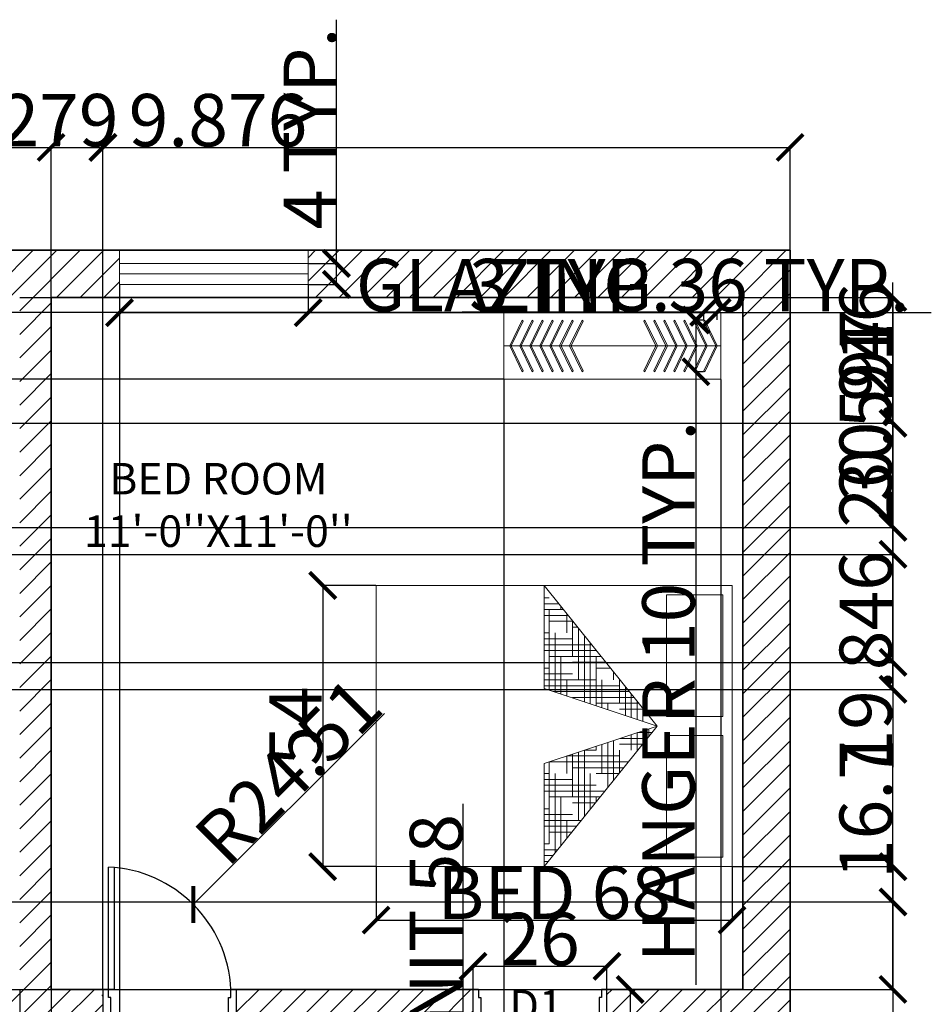
# Model space of a CAD drawing. Units: inches. Extents: x 90933 to 91345, y 21207 to 21646.
# Tile 4 of 4: x 91160 to 91334, y 21458 to 21646. Entities that reach past the tile are written whole.
import ezdxf

# ---------------------------------------------------------------- set-up
doc = ezdxf.new("R2010")
doc.units = ezdxf.units.IN
for name, color, linetype, lineweight in [('A-ANNO-DIMS', 2, 'Continuous', 18), ('A-ANNO-TEXT', 7, 'Continuous', 18), ('A-AREA-IDEN', 7, 'Continuous', 25), ('A-WALL-PATT', 8, 'Continuous', 13), ('B-FURNITURE', 9, 'Continuous', 18), ('Doors', 34, 'Continuous', 25), ('shelves', 42, 'Continuous', 18), ('Walls', 7, 'Continuous', 35), ('Windows', 140, 'Continuous', 18)]:
    doc.layers.add(name, color=color, linetype=linetype, lineweight=lineweight)
doc.styles.get("Standard").update_dxf_attribs({"font": 'arial.ttf'})
doc.dimstyles.get("Standard").update_dxf_attribs({"dimtxt": 10, "dimasz": 5, "dimexe": 0.18, "dimexo": 0.0625, "dimgap": 0.09, "dimtad": 1, "dimdec": 1, "dimzin": 0, "dimdsep": 46, "dimlunit": 4, "dimtxsty": 'Standard', "dimblk": 'ARCHTICK', "dimcen": 0.09, "dimadec": 0, "dimazin": 0, "dimtfac": 1, "dimtdec": 1, "dimtofl": 0, "dimtmove": 0, "dimatfit": 3, "dimldrblk": 'NONE', "dimfxl": 1, "dimtolj": 1, "dimtzin": 0, "dimarcsym": 0})

# ---------------------------------------------------------------- blocks, each defined once
blk = doc.blocks.new('*X5')
at = {"color": 0}
for p, q in [((20.1875, 14.75), (20.1875, 14.7669)), ((20.199, 14.7812), (20.2772, 14.7812)), ((20.25, 14.8125), (20.2772, 14.8125)), ((20.1487, 14.7188), (20.2772, 14.7188)), ((20.1562, 14.625), (20.1562, 14.7281)), ((20.1739, 14.75), (20.2772, 14.75)), ((20.25, 14.3194), (20.25, 14.75)), ((20.0984, 14.6562), (20.125, 14.6562)), ((20.1236, 14.6875), (20.25, 14.6875)), ((20.125, 14.5), (20.125, 14.6893)), ((20.0625, 14.2573), (20.0625, 14.6116)), ((20.0938, 14.375), (20.0938, 14.6504)), ((20.2188, 14.3091), (20.2188, 14.625)), ((20.25, 14.625), (20.2772, 14.625)), ((20.023, 14.5625), (20.2772, 14.5625)), ((20.0312, 14.2469), (20.0312, 14.5727)), ((20.125, 14.5938), (20.2772, 14.5938)), ((19.9727, 14.5), (20.25, 14.5)), ((19.9979, 14.5312), (20.2772, 14.5312)), ((20, 14.2366), (20, 14.5)), ((20.1875, 14.2987), (20.1875, 14.5)), ((19.9476, 14.4688), (20.125, 14.4688)), ((19.9062, 14.375), (19.9062, 14.4174)), ((19.9225, 14.4375), (20, 14.4375)), ((20.125, 14.4062), (20.2772, 14.4062)), ((20.25, 14.4375), (20.2772, 14.4375)), ((19.875, 14.25), (19.875, 14.3785)), ((19.875, 14.3438), (20.2772, 14.3438)), ((19.9688, 14.2262), (19.9688, 14.375)), ((20, 14.375), (20.2772, 14.375)), ((20.1562, 14.2884), (20.1562, 14.375)), ((19.8125, 14.1744), (19.8125, 14.3008)), ((19.8219, 14.3125), (20.2291, 14.3125)), ((19.8438, 14.1848), (19.8438, 14.3397)), ((19.7716, 14.25), (20, 14.25)), ((19.7812, 14.1641), (19.7812, 14.262)), ((19.7967, 14.2812), (20.125, 14.2812)), ((19.9375, 14.2159), (19.9375, 14.25)), ((19.7213, 14.1875), (19.75, 14.1875)), ((19.7465, 14.2188), (19.875, 14.2188)), ((19.75, 14.1537), (19.75, 14.2231)), ((19.7018, 14.0938), (19.7786, 14.0938)), ((19.7188, 14.0726), (19.7188, 14.1136)), ((19.75, 14.0338), (19.75, 14.1032)), ((19.7812, 13.9949), (19.7812, 14.0929)), ((19.8125, 14), (19.8125, 14.0825)), ((19.7269, 14.0625), (19.8728, 14.0625)), ((19.752, 14.0312), (19.875, 14.0312)), ((19.9062, 13.8396), (19.9062, 14.0514)), ((19.9375, 13.8007), (19.9375, 14.0411)), ((19.9688, 13.875), (19.9688, 14.0307)), ((19.875, 13.8784), (19.875, 14)), ((20, 14), (20, 14.0204)), ((20, 14), (20.0614, 14)), ((20.0625, 13.6454), (20.0625, 13.9996)), ((20.0938, 13.625), (20.0938, 13.9893)), ((20.125, 13.75), (20.125, 13.9789)), ((19.8275, 13.9375), (20.25, 13.9375)), ((19.875, 13.9688), (20.1557, 13.9688)), ((20.1562, 13.875), (20.1562, 13.9686)), ((20.25, 13.5), (20.25, 13.9375)), ((19.8526, 13.9062), (20.125, 13.9062)), ((19.8777, 13.875), (20, 13.875)), ((20.0312, 13.6842), (20.0312, 13.875)), ((20.2188, 13.4511), (20.2188, 13.875)), ((20.25, 13.875), (20.2772, 13.875)), ((20.125, 13.8438), (20.2772, 13.8438)), ((19.9532, 13.7812), (20.2772, 13.7812)), ((20, 13.8125), (20.2772, 13.8125)), ((19.9783, 13.75), (20.25, 13.75)), ((20, 13.723), (20, 13.75)), ((20.0035, 13.7188), (20.125, 13.7188)), ((20.1875, 13.49), (20.1875, 13.75)), ((20.25, 13.6875), (20.2772, 13.6875)), ((20.0789, 13.625), (20.2772, 13.625)), ((20.125, 13.6562), (20.2772, 13.6562)), ((20.1562, 13.5288), (20.1562, 13.625)), ((20.104, 13.5938), (20.2772, 13.5938)), ((20.1292, 13.5625), (20.25, 13.5625)), ((20.2046, 13.4688), (20.2772, 13.4688)), ((20.25, 13.5), (20.2772, 13.5)), ((20.2297, 13.4375), (20.2772, 13.4375)), ((20.2549, 13.4062), (20.2772, 13.4062))]:
    blk.add_line(p, q, dxfattribs=at)
blk = doc.blocks.new('MAT-P13')
for p, q in [((-0.75, 0), (0.75, 0)), ((-0.75, 0), (-0.75, -1.9)), ((0.75, 0), (0.75, -1.9)), ((-0.7, -0.05), (-0.7, -0.35)), ((-0.7, -0.05), (-0.05, -0.05)), ((-0.05, -0.35), (-0.05, -0.05)), ((0.05, -0.05), (0.7, -0.05)), ((0.05, -0.35), (0.05, -0.05)), ((0.7, -0.05), (0.7, -0.35)), ((-0.7, -0.35), (-0.05, -0.35)), ((0.05, -0.35), (0.7, -0.35)), ((-0.75, -1.0034), (0, -0.4)), ((0, -0.4), (-0.75, -1.0034)), ((0, -0.4), (-0.2, -1.0034)), ((0, -0.4), (0.2, -1.0034)), ((0, -0.4), (0.75, -1.0034)), ((-0.75, -1.0034), (-0.2, -1.0034)), ((0.2, -1.0034), (0.75, -1.0034)), ((0.75, -1.9), (-0.75, -1.9))]:
    blk.add_line(p, q)
at = {"xscale": -1, "rotation": 90}
blk.add_blockref('*X5', (14.1285, 19.2738), dxfattribs=at)
blk = doc.blocks.new('AP0B05')
for p, q in [((35, 100), (35, 880)), ((75, 100), (75, 878.9))]:
    blk.add_line(p, q)
for points in [[(0, 100), (0, -100), (35, -100), (35, -50), (50, -50), (50, 50), (35, 50), (35, 100)], [(850, 100), (850, -100), (815, -100), (815, -50), (800, -50), (800, 50), (815, 50), (815, 100)]]:
    blk.add_lwpolyline(points, close=True)
blk.add_lwpolyline([(35, 100), (75, 100)])
blk.add_arc((-2.4, 62.6), 818.3, 2.62122, 87.37878)
blk = doc.blocks.new('WARDROBE-HANGER')
for points in [[(0, 4.93), (2.37, 9.86), (2.56, 9.66), (0.27, 4.93)], [(0, 4.93), (2.37, 0), (2.56, 0.21), (0.27, 4.93)]]:
    blk.add_lwpolyline(points)
blk = doc.blocks.new('WINDOW-GLAZING-36IN')
for p, q in [((0, 4), (36, 4)), ((0, 2), (36, 2)), ((0, 0), (36, 0))]:
    blk.add_line(p, q)
blk = doc.blocks.new('_ArchTick')
at = {"color": 0, "linetype": 'ByBlock', "const_width": 0.15}
blk.add_lwpolyline([(-0.5, -0.5), (0.5, 0.5)], dxfattribs=at)
blk = doc.blocks.new('*D16')
at = {"layer": 'A-ANNO-DIMS', "color": 0, "lineweight": -2, "transparency": 16777216}
for p, q in [((91290.56, 21588.31), (91288.96, 21588.31)), ((91289.14, 21588.31), (91289.14, 21578.44)), ((91290.56, 21578.44), (91288.96, 21578.44)), ((91289.14, 21578.44), (91289.14, 21461.47))]:
    blk.add_line(p, q, dxfattribs=at)
at = {"layer": 'Defpoints', "color": 0, "transparency": 16777216}
for p in [(91290.62, 21588.31), (91289.14, 21578.44), (91290.62, 21578.44)]:
    blk.add_point(p, dxfattribs=at)
at = {"layer": 'A-ANNO-DIMS', "color": 0, "lineweight": -2, "transparency": 16777216, "xscale": 5, "yscale": 5, "zscale": 5}
for p, rotation in [((91289.14, 21588.31), 90), ((91289.14, 21578.44), 270)]:
    blk.add_blockref('_ArchTick', p, dxfattribs=dict(at, rotation=rotation))
at = {"layer": 'A-ANNO-DIMS', "color": 0, "transparency": 16777216, "insert": (91283.88, 21517.46), "char_height": 10, "attachment_point": 5, "rotation": 90}
blk.add_mtext('\\A1;HANGER 10 TYP.', dxfattribs=at)
blk = doc.blocks.new('_None')
blk = doc.blocks.new('*D17')
at = {"layer": 'A-ANNO-DIMS', "color": 0, "lineweight": -2, "transparency": 16777216}
for p, q in [((91290.62, 21588.37), (91290.62, 21589.97)), ((91293.18, 21588.37), (91293.18, 21589.97)), ((91290.62, 21589.79), (91244.54, 21589.79)), ((91293.18, 21589.79), (91290.62, 21589.79))]:
    blk.add_line(p, q, dxfattribs=at)
at = {"layer": 'Defpoints', "color": 0, "transparency": 16777216}
for p in [(91290.62, 21589.79), (91290.62, 21588.31), (91293.18, 21588.31)]:
    blk.add_point(p, dxfattribs=at)
at = {"layer": 'A-ANNO-DIMS', "color": 0, "lineweight": -2, "transparency": 16777216, "xscale": 5, "yscale": 5, "zscale": 5, "rotation": 180}
blk.add_blockref('_ArchTick', (91290.62, 21589.79), dxfattribs=at)
at = {"layer": 'A-ANNO-DIMS', "color": 0, "lineweight": -2, "transparency": 16777216, "xscale": 5, "yscale": 5, "zscale": 5}
blk.add_blockref('_ArchTick', (91293.18, 21589.79), dxfattribs=at)
at = {"layer": 'A-ANNO-DIMS', "color": 0, "transparency": 16777216, "insert": (91265.08, 21594.98), "char_height": 10, "attachment_point": 5}
blk.add_mtext('\\A1;3 TYP.', dxfattribs=at)
blk = doc.blocks.new('*D22')
at = {"layer": 'A-ANNO-DIMS', "color": 0, "lineweight": -2, "transparency": 16777216}
for p, q in [((91272.22, 21460.62), (91276.76, 21460.62)), ((91276.58, 21460.62), (91276.58, 21431.16)), ((91272.22, 21431.16), (91276.76, 21431.16)), ((91276.58, 21431.16), (91276.58, 21366.34))]:
    blk.add_line(p, q, dxfattribs=at)
at = {"layer": 'Defpoints', "color": 0, "transparency": 16777216}
for p in [(91272.16, 21460.62), (91272.16, 21431.16), (91276.58, 21431.16)]:
    blk.add_point(p, dxfattribs=at)
at = {"layer": 'A-ANNO-DIMS', "color": 0, "lineweight": -2, "transparency": 16777216, "xscale": 5, "yscale": 5, "zscale": 5}
for p, rotation in [((91276.58, 21460.62), 90), ((91276.58, 21431.16), 270)]:
    blk.add_blockref('_ArchTick', p, dxfattribs=dict(at, rotation=rotation))
at = {"layer": 'A-ANNO-DIMS', "color": 0, "transparency": 16777216, "insert": (91271.31, 21396.25), "char_height": 10, "attachment_point": 5, "rotation": 90}
blk.add_mtext('\\A1;DOOR 29', dxfattribs=at)
blk = doc.blocks.new('*D23')
at = {"layer": 'A-ANNO-DIMS', "color": 0, "lineweight": -2, "transparency": 16777216}
for p, q in [((91246.61, 21460.68), (91246.61, 21465.21)), ((91246.61, 21465.03), (91272.16, 21465.03)), ((91272.16, 21460.68), (91272.16, 21465.21))]:
    blk.add_line(p, q, dxfattribs=at)
at = {"layer": 'Defpoints', "color": 0, "transparency": 16777216}
for p in [(91272.16, 21465.03), (91246.61, 21460.62), (91272.16, 21460.62)]:
    blk.add_point(p, dxfattribs=at)
at = {"layer": 'A-ANNO-DIMS', "color": 0, "lineweight": -2, "transparency": 16777216, "xscale": 5, "yscale": 5, "zscale": 5, "rotation": 180}
blk.add_blockref('_ArchTick', (91246.61, 21465.03), dxfattribs=at)
at = {"layer": 'A-ANNO-DIMS', "color": 0, "lineweight": -2, "transparency": 16777216, "xscale": 5, "yscale": 5, "zscale": 5}
blk.add_blockref('_ArchTick', (91272.16, 21465.03), dxfattribs=at)
at = {"layer": 'A-ANNO-DIMS', "color": 0, "transparency": 16777216, "insert": (91259.39, 21470.23), "char_height": 10, "attachment_point": 5}
blk.add_mtext('\\A1;26', dxfattribs=at)
blk = doc.blocks.new('*D26')
at = {"layer": 'A-ANNO-DIMS', "color": 0, "lineweight": -2, "transparency": 16777216}
for p, q in [((91179.14, 21595.05), (91179.14, 21589.54)), ((91215.14, 21595.05), (91215.14, 21589.54)), ((91179.14, 21589.72), (91215.14, 21589.72)), ((91215.14, 21589.72), (91334.04, 21589.72))]:
    blk.add_line(p, q, dxfattribs=at)
at = {"layer": 'Defpoints', "color": 0, "transparency": 16777216}
for p in [(91179.14, 21595.12), (91215.14, 21595.12), (91215.14, 21589.72)]:
    blk.add_point(p, dxfattribs=at)
at = {"layer": 'A-ANNO-DIMS', "color": 0, "lineweight": -2, "transparency": 16777216, "xscale": 5, "yscale": 5, "zscale": 5, "rotation": 180}
blk.add_blockref('_ArchTick', (91179.14, 21589.72), dxfattribs=at)
at = {"layer": 'A-ANNO-DIMS', "color": 0, "lineweight": -2, "transparency": 16777216, "xscale": 5, "yscale": 5, "zscale": 5}
blk.add_blockref('_ArchTick', (91215.14, 21589.72), dxfattribs=at)
at = {"layer": 'A-ANNO-DIMS', "color": 0, "transparency": 16777216, "insert": (91277.09, 21594.98), "char_height": 10, "attachment_point": 5}
blk.add_mtext('\\A1;GLAZING 36 TYP.', dxfattribs=at)
blk = doc.blocks.new('*D27')
at = {"layer": 'A-ANNO-DIMS', "color": 0, "lineweight": -2, "transparency": 16777216}
for p, q in [((91220.54, 21599.12), (91220.54, 21645.61)), ((91215.21, 21599.12), (91220.72, 21599.12)), ((91220.54, 21595.12), (91220.54, 21599.12)), ((91215.21, 21595.12), (91220.72, 21595.12))]:
    blk.add_line(p, q, dxfattribs=at)
at = {"layer": 'Defpoints', "color": 0, "transparency": 16777216}
for p in [(91215.14, 21599.12), (91220.54, 21599.12), (91215.14, 21595.12)]:
    blk.add_point(p, dxfattribs=at)
at = {"layer": 'A-ANNO-DIMS', "color": 0, "lineweight": -2, "transparency": 16777216, "xscale": 5, "yscale": 5, "zscale": 5}
for p, rotation in [((91220.54, 21599.12), 90), ((91220.54, 21595.12), 270)]:
    blk.add_blockref('_ArchTick', p, dxfattribs=dict(at, rotation=rotation))
at = {"layer": 'A-ANNO-DIMS', "color": 0, "transparency": 16777216, "insert": (91215.45, 21624.86), "char_height": 10, "attachment_point": 5, "rotation": 90}
blk.add_mtext('\\A1;4 TYP.', dxfattribs=at)
blk = doc.blocks.new('*D30')
at = {"layer": 'A-ANNO-DIMS', "color": 0, "lineweight": -2, "transparency": 16777216}
for p, q in [((91228.11, 21483.99), (91228.11, 21473.68)), ((91296.04, 21483.99), (91296.04, 21473.68)), ((91228.11, 21473.86), (91296.04, 21473.86))]:
    blk.add_line(p, q, dxfattribs=at)
at = {"layer": 'Defpoints', "color": 0, "transparency": 16777216}
for p in [(91228.11, 21484.05), (91296.04, 21484.05), (91296.04, 21473.86)]:
    blk.add_point(p, dxfattribs=at)
at = {"layer": 'A-ANNO-DIMS', "color": 0, "lineweight": -2, "transparency": 16777216, "xscale": 5, "yscale": 5, "zscale": 5, "rotation": 180}
blk.add_blockref('_ArchTick', (91228.11, 21473.86), dxfattribs=at)
at = {"layer": 'A-ANNO-DIMS', "color": 0, "lineweight": -2, "transparency": 16777216, "xscale": 5, "yscale": 5, "zscale": 5}
blk.add_blockref('_ArchTick', (91296.04, 21473.86), dxfattribs=at)
at = {"layer": 'A-ANNO-DIMS', "color": 0, "transparency": 16777216, "insert": (91262.08, 21479.06), "char_height": 10, "attachment_point": 5}
blk.add_mtext('\\A1;BED 68', dxfattribs=at)
blk = doc.blocks.new('*D31')
at = {"layer": 'A-ANNO-DIMS', "color": 0, "lineweight": -2, "transparency": 16777216}
for p, q in [((91228.05, 21537.68), (91217.74, 21537.68)), ((91217.92, 21537.68), (91217.92, 21484.05)), ((91228.05, 21484.05), (91217.74, 21484.05))]:
    blk.add_line(p, q, dxfattribs=at)
at = {"layer": 'Defpoints', "color": 0, "transparency": 16777216}
for p in [(91228.11, 21537.68), (91217.92, 21484.05), (91228.11, 21484.05)]:
    blk.add_point(p, dxfattribs=at)
at = {"layer": 'A-ANNO-DIMS', "color": 0, "lineweight": -2, "transparency": 16777216, "xscale": 5, "yscale": 5, "zscale": 5}
for p, rotation in [((91217.92, 21537.68), 90), ((91217.92, 21484.05), 270)]:
    blk.add_blockref('_ArchTick', p, dxfattribs=dict(at, rotation=rotation))
at = {"layer": 'A-ANNO-DIMS', "color": 0, "transparency": 16777216, "insert": (91212.74, 21510.87), "char_height": 10, "attachment_point": 5, "rotation": 90}
blk.add_mtext('\\A1;54', dxfattribs=at)
blk = doc.blocks.new('*D36')
at = {"layer": 'A-ANNO-DIMS', "color": 0, "lineweight": -2, "transparency": 16777216}
for p, q in [((91244.73, 21418.04), (91244.73, 21496.03)), ((91236.1, 21418.04), (91244.91, 21418.04)), ((91244.73, 21360.1), (91244.73, 21418.04)), ((91236.1, 21360.1), (91244.91, 21360.1))]:
    blk.add_line(p, q, dxfattribs=at)
at = {"layer": 'Defpoints', "color": 0, "transparency": 16777216}
for p in [(91236.04, 21418.04), (91244.73, 21418.04), (91236.04, 21360.1)]:
    blk.add_point(p, dxfattribs=at)
at = {"layer": 'A-ANNO-DIMS', "color": 0, "lineweight": -2, "transparency": 16777216, "xscale": 5, "yscale": 5, "zscale": 5}
for p, rotation in [((91244.73, 21418.04), 90), ((91244.73, 21360.1), 270)]:
    blk.add_blockref('_ArchTick', p, dxfattribs=dict(at, rotation=rotation))
at = {"layer": 'A-ANNO-DIMS', "color": 0, "transparency": 16777216, "insert": (91239.53, 21459.53), "char_height": 10, "attachment_point": 5, "rotation": 90}
blk.add_mtext('\\A1;TV UNIT 58', dxfattribs=at)
blk = doc.blocks.new('*D41')
at = {"layer": 'A-ANNO-DIMS', "color": 0, "lineweight": -2, "transparency": 16777216}
for p, q in [((91166.1, 21592.55), (91166.1, 21209.81)), ((91179.14, 21592.55), (91179.14, 21209.81)), ((91166.1, 21209.99), (91179.14, 21209.99)), ((91179.14, 21209.99), (91224.86, 21209.99))]:
    blk.add_line(p, q, dxfattribs=at)
at = {"layer": 'Defpoints', "color": 0, "transparency": 16777216}
for p in [(91166.1, 21592.62), (91179.14, 21592.62), (91179.14, 21209.99)]:
    blk.add_point(p, dxfattribs=at)
at = {"layer": 'A-ANNO-DIMS', "color": 0, "lineweight": -2, "transparency": 16777216, "xscale": 5, "yscale": 5, "zscale": 5, "rotation": 180}
blk.add_blockref('_ArchTick', (91166.1, 21209.99), dxfattribs=at)
at = {"layer": 'A-ANNO-DIMS', "color": 0, "lineweight": -2, "transparency": 16777216, "xscale": 5, "yscale": 5, "zscale": 5}
blk.add_blockref('_ArchTick', (91179.14, 21209.99), dxfattribs=at)
at = {"layer": 'A-ANNO-DIMS', "color": 0, "transparency": 16777216, "insert": (91204.5, 21215.18), "char_height": 10, "attachment_point": 5}
blk.add_mtext('\\A1;13.044', dxfattribs=at)
blk = doc.blocks.new('*D49')
at = {"layer": 'A-ANNO-DIMS', "color": 0, "lineweight": -2, "transparency": 16777216}
for p, q in [((91160.1, 21460.55), (91160.1, 21209.81)), ((91142.5, 21454.55), (91142.5, 21209.81)), ((91142.5, 21209.99), (91160.1, 21209.99)), ((91160.1, 21209.99), (91205.85, 21209.99))]:
    blk.add_line(p, q, dxfattribs=at)
at = {"layer": 'Defpoints', "color": 0, "transparency": 16777216}
for p in [(91160.1, 21460.62), (91142.5, 21454.62), (91160.1, 21209.99)]:
    blk.add_point(p, dxfattribs=at)
at = {"layer": 'A-ANNO-DIMS', "color": 0, "lineweight": -2, "transparency": 16777216, "xscale": 5, "yscale": 5, "zscale": 5, "rotation": 180}
blk.add_blockref('_ArchTick', (91142.5, 21209.99), dxfattribs=at)
at = {"layer": 'A-ANNO-DIMS', "color": 0, "lineweight": -2, "transparency": 16777216, "xscale": 5, "yscale": 5, "zscale": 5}
blk.add_blockref('_ArchTick', (91160.1, 21209.99), dxfattribs=at)
at = {"layer": 'A-ANNO-DIMS', "color": 0, "transparency": 16777216, "insert": (91185.47, 21215.18), "char_height": 10, "attachment_point": 5}
blk.add_mtext('\\A1;17.596', dxfattribs=at)
blk = doc.blocks.new('*D50')
at = {"layer": 'A-ANNO-DIMS', "color": 0, "lineweight": -2, "transparency": 16777216}
for p, q in [((91166.1, 21460.68), (91166.1, 21621.43)), ((91166.1, 21621.25), (91175.98, 21621.25)), ((91175.98, 21460.67), (91175.98, 21621.43)), ((91175.98, 21621.25), (91214.89, 21621.25))]:
    blk.add_line(p, q, dxfattribs=at)
at = {"layer": 'Defpoints', "color": 0, "transparency": 16777216}
for p in [(91175.98, 21621.25), (91166.1, 21460.62), (91175.98, 21460.61)]:
    blk.add_point(p, dxfattribs=at)
at = {"layer": 'A-ANNO-DIMS', "color": 0, "lineweight": -2, "transparency": 16777216, "xscale": 5, "yscale": 5, "zscale": 5, "rotation": 180}
blk.add_blockref('_ArchTick', (91166.1, 21621.25), dxfattribs=at)
at = {"layer": 'A-ANNO-DIMS', "color": 0, "lineweight": -2, "transparency": 16777216, "xscale": 5, "yscale": 5, "zscale": 5}
blk.add_blockref('_ArchTick', (91175.98, 21621.25), dxfattribs=at)
at = {"layer": 'A-ANNO-DIMS', "color": 0, "transparency": 16777216, "insert": (91197.94, 21626.44), "char_height": 10, "attachment_point": 5}
blk.add_mtext('\\A1;9.876', dxfattribs=at)
blk = doc.blocks.new('*D53')
at = {"layer": 'A-ANNO-DIMS', "color": 0, "lineweight": -2, "transparency": 16777216}
for p, q in [((91160.1, 21460.55), (91160.1, 21209.81)), ((91166.1, 21460.55), (91166.1, 21209.81)), ((91160.1, 21209.99), (91166.1, 21209.99)), ((91166.1, 21209.99), (91177.88, 21209.99))]:
    blk.add_line(p, q, dxfattribs=at)
at = {"layer": 'Defpoints', "color": 0, "transparency": 16777216}
for p in [(91160.1, 21460.62), (91166.1, 21460.62), (91166.1, 21209.99)]:
    blk.add_point(p, dxfattribs=at)
at = {"layer": 'A-ANNO-DIMS', "color": 0, "lineweight": -2, "transparency": 16777216, "xscale": 5, "yscale": 5, "zscale": 5, "rotation": 180}
blk.add_blockref('_ArchTick', (91160.1, 21209.99), dxfattribs=at)
at = {"layer": 'A-ANNO-DIMS', "color": 0, "lineweight": -2, "transparency": 16777216, "xscale": 5, "yscale": 5, "zscale": 5}
blk.add_blockref('_ArchTick', (91166.1, 21209.99), dxfattribs=at)
at = {"layer": 'A-ANNO-DIMS', "color": 0, "transparency": 16777216, "insert": (91174.49, 21215.18), "char_height": 10, "attachment_point": 5}
blk.add_mtext('\\A1;6', dxfattribs=at)
blk = doc.blocks.new('*D59')
at = {"layer": 'A-ANNO-DIMS', "color": 0, "lineweight": -2, "transparency": 16777216}
for p, q in [((91326.73, 21548.77), (91326.73, 21595.45)), ((91057.49, 21548.77), (91326.91, 21548.77)), ((91326.73, 21517.85), (91326.73, 21548.77)), ((91057.49, 21517.85), (91326.91, 21517.85))]:
    blk.add_line(p, q, dxfattribs=at)
at = {"layer": 'Defpoints', "color": 0, "transparency": 16777216}
for p in [(91057.43, 21548.77), (91326.73, 21548.77), (91057.43, 21517.85)]:
    blk.add_point(p, dxfattribs=at)
at = {"layer": 'A-ANNO-DIMS', "color": 0, "lineweight": -2, "transparency": 16777216, "xscale": 5, "yscale": 5, "zscale": 5}
for p, rotation in [((91326.73, 21548.77), 90), ((91326.73, 21517.85), 270)]:
    blk.add_blockref('_ArchTick', p, dxfattribs=dict(at, rotation=rotation))
at = {"layer": 'A-ANNO-DIMS', "color": 0, "transparency": 16777216, "insert": (91321.53, 21574.61), "char_height": 10, "attachment_point": 5, "rotation": 90}
blk.add_mtext('\\A1;30.916', dxfattribs=at)
blk = doc.blocks.new('*D62')
at = {"layer": 'A-ANNO-DIMS', "color": 0, "lineweight": -2, "transparency": 16777216}
for p, q in [((91252.49, 21576.95), (91252.49, 21209.81)), ((91293.88, 21576.95), (91293.88, 21209.81)), ((91252.49, 21209.99), (91293.88, 21209.99))]:
    blk.add_line(p, q, dxfattribs=at)
at = {"layer": 'Defpoints', "color": 0, "transparency": 16777216}
for p in [(91252.49, 21577.01), (91293.88, 21577.01), (91293.88, 21209.99)]:
    blk.add_point(p, dxfattribs=at)
at = {"layer": 'A-ANNO-DIMS', "color": 0, "lineweight": -2, "transparency": 16777216, "xscale": 5, "yscale": 5, "zscale": 5, "rotation": 180}
blk.add_blockref('_ArchTick', (91252.49, 21209.99), dxfattribs=at)
at = {"layer": 'A-ANNO-DIMS', "color": 0, "lineweight": -2, "transparency": 16777216, "xscale": 5, "yscale": 5, "zscale": 5}
blk.add_blockref('_ArchTick', (91293.88, 21209.99), dxfattribs=at)
at = {"layer": 'A-ANNO-DIMS', "color": 0, "transparency": 16777216, "insert": (91273.18, 21215.18), "char_height": 10, "attachment_point": 5}
blk.add_mtext('\\A1;41.38', dxfattribs=at)
blk = doc.blocks.new('*D63')
at = {"layer": 'A-ANNO-DIMS', "color": 0, "lineweight": -2, "transparency": 16777216}
for p, q in [((91008.47, 21589.73), (91008.47, 21635.49)), ((91252.43, 21589.73), (91008.29, 21589.73)), ((91008.47, 21577.01), (91008.47, 21589.73)), ((91252.43, 21577.01), (91008.29, 21577.01))]:
    blk.add_line(p, q, dxfattribs=at)
at = {"layer": 'Defpoints', "color": 0, "transparency": 16777216}
for p in [(91008.47, 21589.73), (91252.49, 21589.73), (91252.49, 21577.01)]:
    blk.add_point(p, dxfattribs=at)
at = {"layer": 'A-ANNO-DIMS', "color": 0, "lineweight": -2, "transparency": 16777216, "xscale": 5, "yscale": 5, "zscale": 5}
for p, rotation in [((91008.47, 21589.73), 90), ((91008.47, 21577.01), 270)]:
    blk.add_blockref('_ArchTick', p, dxfattribs=dict(at, rotation=rotation))
at = {"layer": 'A-ANNO-DIMS', "color": 0, "transparency": 16777216, "insert": (91003.36, 21615.11), "char_height": 10, "attachment_point": 5, "rotation": 90}
blk.add_mtext('\\A1;12.717', dxfattribs=at)
blk = doc.blocks.new('*D64')
at = {"layer": 'A-ANNO-DIMS', "color": 0, "lineweight": -2, "transparency": 16777216}
for p, q in [((91028.1, 21601.68), (91028.1, 21621.43)), ((91028.1, 21621.25), (91307.1, 21621.25)), ((91307.1, 21601.68), (91307.1, 21621.43))]:
    blk.add_line(p, q, dxfattribs=at)
at = {"layer": 'Defpoints', "color": 0, "transparency": 16777216}
for p in [(91307.1, 21621.25), (91028.1, 21601.62), (91307.1, 21601.62)]:
    blk.add_point(p, dxfattribs=at)
at = {"layer": 'A-ANNO-DIMS', "color": 0, "lineweight": -2, "transparency": 16777216, "xscale": 5, "yscale": 5, "zscale": 5, "rotation": 180}
blk.add_blockref('_ArchTick', (91028.1, 21621.25), dxfattribs=at)
at = {"layer": 'A-ANNO-DIMS', "color": 0, "lineweight": -2, "transparency": 16777216, "xscale": 5, "yscale": 5, "zscale": 5}
blk.add_blockref('_ArchTick', (91307.1, 21621.25), dxfattribs=at)
at = {"layer": 'A-ANNO-DIMS', "color": 0, "transparency": 16777216, "insert": (91167.6, 21626.44), "char_height": 10, "attachment_point": 5}
blk.add_mtext('\\A1;279', dxfattribs=at)
blk = doc.blocks.new('*D66')
at = {"layer": 'A-ANNO-DIMS', "color": 0, "lineweight": -2, "transparency": 16777216}
for p, q in [((91061.16, 21568.62), (91326.91, 21568.62)), ((91326.73, 21568.62), (91326.73, 21548.77)), ((91057.49, 21548.77), (91326.91, 21548.77)), ((91326.73, 21548.77), (91326.73, 21503.02))]:
    blk.add_line(p, q, dxfattribs=at)
at = {"layer": 'Defpoints', "color": 0, "transparency": 16777216}
for p in [(91061.1, 21568.62), (91057.43, 21548.77), (91326.73, 21548.77)]:
    blk.add_point(p, dxfattribs=at)
at = {"layer": 'A-ANNO-DIMS', "color": 0, "lineweight": -2, "transparency": 16777216, "xscale": 5, "yscale": 5, "zscale": 5}
for p, rotation in [((91326.73, 21568.62), 90), ((91326.73, 21548.77), 270)]:
    blk.add_blockref('_ArchTick', p, dxfattribs=dict(at, rotation=rotation))
at = {"layer": 'A-ANNO-DIMS', "color": 0, "transparency": 16777216, "insert": (91321.53, 21523.4), "char_height": 10, "attachment_point": 5, "rotation": 90}
blk.add_mtext('\\A1;19.846', dxfattribs=at)
blk = doc.blocks.new('*D67')
at = {"layer": 'A-ANNO-DIMS', "color": 0, "lineweight": -2, "transparency": 16777216}
for p, q in [((91326.73, 21477.31), (91326.73, 21507.53)), ((91057.47, 21477.31), (91326.91, 21477.31)), ((91326.73, 21460.62), (91326.73, 21477.31)), ((91061.16, 21460.62), (91326.91, 21460.62))]:
    blk.add_line(p, q, dxfattribs=at)
at = {"layer": 'Defpoints', "color": 0, "transparency": 16777216}
for p in [(91057.41, 21477.31), (91326.73, 21477.31), (91061.1, 21460.62)]:
    blk.add_point(p, dxfattribs=at)
at = {"layer": 'A-ANNO-DIMS', "color": 0, "lineweight": -2, "transparency": 16777216, "xscale": 5, "yscale": 5, "zscale": 5}
for p, rotation in [((91326.73, 21477.31), 90), ((91326.73, 21460.62), 270)]:
    blk.add_blockref('_ArchTick', p, dxfattribs=dict(at, rotation=rotation))
at = {"layer": 'A-ANNO-DIMS', "color": 0, "transparency": 16777216, "insert": (91321.53, 21494.92), "char_height": 10, "attachment_point": 5, "rotation": 90}
blk.add_mtext('\\A1;16.7', dxfattribs=at)
blk = doc.blocks.new('*D68')
at = {"layer": 'A-ANNO-DIMS', "color": 0, "lineweight": -2, "transparency": 16777216}
for p, q in [((91296.1, 21484.05), (91326.91, 21484.05)), ((91326.73, 21484.05), (91326.73, 21460.62)), ((91298.16, 21460.62), (91326.91, 21460.62)), ((91326.73, 21460.62), (91326.73, 21413.73))]:
    blk.add_line(p, q, dxfattribs=at)
at = {"layer": 'Defpoints', "color": 0, "transparency": 16777216}
for p in [(91296.04, 21484.05), (91298.1, 21460.62), (91326.73, 21460.62)]:
    blk.add_point(p, dxfattribs=at)
at = {"layer": 'A-ANNO-DIMS', "color": 0, "lineweight": -2, "transparency": 16777216, "xscale": 5, "yscale": 5, "zscale": 5}
for p, rotation in [((91326.73, 21484.05), 90), ((91326.73, 21460.62), 270)]:
    blk.add_blockref('_ArchTick', p, dxfattribs=dict(at, rotation=rotation))
at = {"layer": 'A-ANNO-DIMS', "color": 0, "transparency": 16777216, "insert": (91321.53, 21434.67), "char_height": 10, "attachment_point": 5, "rotation": 90}
blk.add_mtext('\\A1;23.438', dxfattribs=at)
blk = doc.blocks.new('*D70')
at = {"layer": 'A-ANNO-DIMS', "color": 0, "lineweight": -2, "transparency": 16777216}
for p, q in [((91160.16, 21592.62), (91326.91, 21592.62)), ((91326.73, 21592.62), (91326.73, 21568.62)), ((91160.16, 21568.62), (91326.91, 21568.62))]:
    blk.add_line(p, q, dxfattribs=at)
at = {"layer": 'Defpoints', "color": 0, "transparency": 16777216}
for p in [(91160.1, 21592.62), (91160.1, 21568.62), (91326.73, 21568.62)]:
    blk.add_point(p, dxfattribs=at)
at = {"layer": 'A-ANNO-DIMS', "color": 0, "lineweight": -2, "transparency": 16777216, "xscale": 5, "yscale": 5, "zscale": 5}
for p, rotation in [((91326.73, 21592.62), 90), ((91326.73, 21568.62), 270)]:
    blk.add_blockref('_ArchTick', p, dxfattribs=dict(at, rotation=rotation))
at = {"layer": 'A-ANNO-DIMS', "color": 0, "transparency": 16777216, "insert": (91321.62, 21580.62), "char_height": 10, "attachment_point": 5, "rotation": 90}
blk.add_mtext('\\A1;24', dxfattribs=at)
blk = doc.blocks.new('*D72')
at = {"layer": 'A-ANNO-DIMS', "color": 0, "lineweight": -2, "transparency": 16777216}
for p, q in [((91326.73, 21543.61), (91326.73, 21590.47)), ((91052.65, 21543.61), (91326.91, 21543.61)), ((91326.73, 21523.01), (91326.73, 21543.61)), ((91052.65, 21523.01), (91326.91, 21523.01))]:
    blk.add_line(p, q, dxfattribs=at)
at = {"layer": 'Defpoints', "color": 0, "transparency": 16777216}
for p in [(91052.59, 21543.61), (91326.73, 21543.61), (91052.59, 21523.01)]:
    blk.add_point(p, dxfattribs=at)
at = {"layer": 'A-ANNO-DIMS', "color": 0, "lineweight": -2, "transparency": 16777216, "xscale": 5, "yscale": 5, "zscale": 5}
for p, rotation in [((91326.73, 21543.61), 90), ((91326.73, 21523.01), 270)]:
    blk.add_blockref('_ArchTick', p, dxfattribs=dict(at, rotation=rotation))
at = {"layer": 'A-ANNO-DIMS', "color": 0, "transparency": 16777216, "insert": (91321.53, 21569.54), "char_height": 10, "attachment_point": 5, "rotation": 90}
blk.add_mtext('\\A1;20.597', dxfattribs=at)
blk = doc.blocks.new('*D79')
at = {"layer": 'A-ANNO-DIMS', "color": 0, "lineweight": -2, "transparency": 16777216}
for p, q in [((91229.69, 21513.28), (91193.23, 21476.82)), ((91175.81, 21459.48), (91175.99, 21459.48)), ((91175.9, 21459.39), (91175.9, 21459.57))]:
    blk.add_line(p, q, dxfattribs=at)
at = {"layer": 'Defpoints', "color": 0, "transparency": 16777216}
for p in [(91193.23, 21476.82), (91175.9, 21459.48)]:
    blk.add_point(p, dxfattribs=at)
at = {"layer": 'A-ANNO-DIMS', "color": 0, "lineweight": -2, "transparency": 16777216, "xscale": 5, "yscale": 5, "zscale": 5, "rotation": 225.0007438936674}
blk.add_blockref('_ArchTick', (91193.23, 21476.82), dxfattribs=at)
at = {"layer": 'A-ANNO-DIMS', "color": 0, "transparency": 16777216, "insert": (91211.33, 21502.26), "char_height": 10, "attachment_point": 5, "rotation": 45.0007}
blk.add_mtext('\\A1;R24.51', dxfattribs=at)

msp = doc.modelspace()

# ---------------------------------------------------------------- hatches: boundary and pattern name
at = {"layer": 'A-WALL-PATT', "transparency": 33554585}
h = msp.add_hatch(dxfattribs=at)
h.set_pattern_fill('ANSI31', color=256)
h.paths.add_polyline_path([(91179.1445, 21601.6157), (91028.1004, 21601.6157), (91028.1004, 21515.2814), (91037.1004, 21515.2814), (91037.1004, 21592.6157), (91160.1004, 21592.6157), (91160.1004, 21460.6157), (91142.5048, 21460.6157), (91142.5048, 21454.6157), (91175.976, 21454.6157), (91175.976, 21460.6157), (91166.1004, 21460.6157), (91166.1004, 21592.6157), (91179.1445, 21592.6157)])
h.paths.add_polyline_path([(91307.1004, 21601.6157), (91215.1445, 21601.6157), (91215.1445, 21592.6157), (91298.1004, 21592.6157), (91298.1004, 21460.6157), (91272.1605, 21460.6157), (91272.1605, 21454.6157), (91298.1004, 21454.6157), (91298.1004, 21384.4519), (91307.1004, 21384.4519)])
h.paths.add_polyline_path([(91037.1004, 21454.6157), (91086.5447, 21454.6157), (91086.5447, 21460.6157), (91037.1004, 21460.6157), (91037.1004, 21479.2814), (91028.1004, 21479.2814), (91028.1004, 21412.6157), (91037.1004, 21412.6157)])
h.paths.add_polyline_path([(91307.1004, 21348.4519), (91298.1004, 21348.4519), (91298.1004, 21322.6157), (91244.1004, 21322.6157), (91244.1004, 21454.6157), (91246.6116, 21454.6157), (91246.6116, 21460.6157), (91201.4342, 21460.6157), (91201.4342, 21454.6157), (91238.1004, 21454.6157), (91238.1004, 21322.6157), (91160.7949, 21322.6157), (91160.7949, 21316.6157), (91298.1004, 21316.6157), (91298.1004, 21238.6157), (91160.1004, 21238.6157), (91160.1004, 21229.6157), (91307.1004, 21229.6157)])
h.paths.add_polyline_path([(91037.1004, 21316.6157), (91049.0004, 21316.6157), (91049.0004, 21322.6157), (91037.1004, 21322.6157), (91037.1004, 21364.6157), (91028.1004, 21364.6157), (91028.1004, 21229.6157), (91037.1004, 21229.6157)])
h.paths.add_polyline_path([(91112.7949, 21322.6157), (91074.4445, 21322.6157), (91074.4445, 21316.6157), (91112.7949, 21316.6157)])

# ---------------------------------------------------------------- linework, layer by layer
at = {"layer": 'shelves'}
msp.add_line((91252.4937, 21583.3737), (91293.8759, 21583.3737), dxfattribs=at)
msp.add_lwpolyline([(91252.4937, 21589.7325), (91293.8759, 21589.7325), (91293.8759, 21577.015), (91252.4937, 21577.015)], close=True, dxfattribs=at)
at = {"layer": 'Walls'}
for p, q in [((91028.1004, 21601.6157), (91307.1004, 21601.6157)), ((91307.1004, 21601.6157), (91307.1004, 21229.6157)), ((91166.1004, 21592.6157), (91166.1004, 21460.6157)), ((91166.1004, 21592.6157), (91298.1004, 21592.6157)), ((91298.1004, 21592.6157), (91298.1004, 21460.6157)), ((91166.1004, 21460.6157), (91178.2223, 21460.6157)), ((91200.3854, 21460.6157), (91247.6636, 21460.6157)), ((91271.1085, 21460.6157), (91298.1004, 21460.6157))]:
    msp.add_line(p, q, dxfattribs=at)
at = {"layer": 'Windows'}
msp.add_lwpolyline([(91179.1445, 21601.6157), (91215.1445, 21601.6157), (91215.1445, 21592.6157), (91179.1445, 21592.6157)], close=True, dxfattribs=at)

# ---------------------------------------------------------------- block references
at = {"layer": 'B-FURNITURE', "xscale": 35.75449165397885, "yscale": 35.75449165397885, "zscale": 35.75449165397885, "rotation": 270}
msp.add_blockref('MAT-P13', (91296.0425, 21510.8691), dxfattribs=at)
at = {"layer": 'Doors', "xscale": 0.0299507821919959, "yscale": 0.0299507821919959, "zscale": 0.0299507821919959}
msp.add_blockref('AP0B05', (91175.976, 21457.6107), dxfattribs=at)
at = {"layer": 'Doors', "xscale": -0.0300575518172249, "yscale": 0.0300575518172249, "zscale": 0.0300575518172249, "rotation": 180}
msp.add_blockref('AP0B05', (91246.6116, 21457.6099), dxfattribs=at)
at = {"layer": 'shelves'}
for p in [(91253.625, 21578.442), (91255.5259, 21578.442), (91257.4267, 21578.442), (91259.3276, 21578.442), (91261.2285, 21578.442), (91263.1293, 21578.442), (91265.0302, 21578.442)]:
    msp.add_blockref('WARDROBE-HANGER', p, dxfattribs=at)
at = {"layer": 'shelves', "rotation": 180}
for p in [(91281.7775, 21588.3055), (91283.6784, 21588.3055), (91285.5793, 21588.3055), (91287.4801, 21588.3055), (91289.381, 21588.3055), (91291.2819, 21588.3055), (91293.1827, 21588.3055)]:
    msp.add_blockref('WARDROBE-HANGER', p, dxfattribs=at)
at = {"layer": 'Windows'}
msp.add_blockref('WINDOW-GLAZING-36IN', (91179.145, 21595.116), dxfattribs=at)

# ---------------------------------------------------------------- texts
at = {"layer": 'A-ANNO-TEXT'}
msp.add_text('D1', height=6, dxfattribs=at).set_placement((91253.5575, 21454.5376))
at = {"layer": 'A-AREA-IDEN', "insert": (91174.9146, 21561.0421), "char_height": 6, "attachment_point": 1}
msp.add_mtext_dynamic_manual_height_columns("\\pxqc;BED ROOM\\P11'-0''X11'-0''", width=46.179351, gutter_width=12.5, heights=[0], dxfattribs=at)

# ---------------------------------------------------------------- dimensions: what is measured, and where the dimension line sits
at = {"layer": 'A-ANNO-DIMS'}
for base, p1, p2, angle, text, picture, middle in [((91220.5445, 21599.1157), (91215.1445, 21595.1157), (91215.1445, 21599.1157), 90, '<> TYP.', '*D27', (91215.4511, 21624.8605)), ((91290.6242, 21589.7851), (91293.1825, 21588.3056), (91290.6242, 21588.3056), 180, '<> TYP.', '*D17', (91265.084, 21594.9843)), ((91289.1447, 21578.4419), (91290.6242, 21588.3056), (91290.6242, 21578.4419), 270, 'HANGER <> TYP.', '*D16', (91283.8841, 21517.4583)), ((91244.7276, 21418.0428), (91236.0368, 21360.1043), (91236.0368, 21418.0428), 90, 'TV UNIT <>', '*D36', (91239.5318, 21459.5345)), ((91276.5789, 21431.1593), (91272.1605, 21460.6157), (91272.1605, 21431.1593), 270, 'DOOR <>', '*D22', (91271.315, 21396.25))]:
    dim = msp.add_linear_dim(base=base, p1=p1, p2=p2, angle=angle, text=text, dimstyle='Standard', override={"dimdec": 0, "dimlfac": 1, "dimrnd": 0, "dimzin": 0, "dimdsep": 46, "dimlunit": 2}, dxfattribs=at)
    dim.commit()
    dim.dimension.update_dxf_attribs({"geometry": picture, "text_midpoint": middle})
for base, p1, p2, angle, override, picture, middle in [((91008.47045, 21589.73247), (91252.49375, 21577.015), (91252.49375, 21589.73247), 90, {"dimdec": 3, "dimlfac": 1, "dimrnd": 0, "dimzin": 0, "dimdsep": 46, "dimlunit": 2}, '*D63', (91003.35999, 21615.10897)), ((91326.7305, 21548.7693), (91057.426, 21517.8533), (91057.426, 21548.7693), 90, {"dimdec": 3, "dimlfac": 1, "dimrnd": 0, "dimzin": 0, "dimdsep": 46, "dimlunit": 2}, '*D59', (91321.5313, 21574.6097)), ((91326.7305, 21568.6157), (91160.1004, 21592.6157), (91160.1004, 21568.6157), 90, {"dimdec": 0, "dimlfac": 1, "dimrnd": 0, "dimzin": 0, "dimdsep": 46, "dimlunit": 2}, '*D70', (91321.62, 21580.6157)), ((91326.7305, 21543.61), (91052.5895, 21523.0127), (91052.5895, 21543.61), 90, {"dimdec": 3, "dimlfac": 1, "dimrnd": 0, "dimzin": 0, "dimdsep": 46, "dimlunit": 2}, '*D72', (91321.5347, 21569.5424)), ((91326.7305, 21548.7693), (91061.1004, 21568.6157), (91057.426, 21548.7693), 90, {"dimdec": 3, "dimlfac": 1, "dimrnd": 0, "dimzin": 0, "dimdsep": 46, "dimlunit": 2}, '*D66', (91321.5347, 21523.3962)), ((91217.9189, 21484.0532), (91228.109, 21537.685), (91228.109, 21484.0532), 270, {"dimdec": 0, "dimlfac": 1, "dimrnd": 0, "dimzin": 0, "dimdsep": 46, "dimlunit": 2}, '*D31', (91212.7437, 21510.8691)), ((91326.7305, 21477.3143), (91061.1004, 21460.6157), (91057.4101, 21477.3143), 90, {"dimdec": 1, "dimlfac": 1, "dimrnd": 0, "dimzin": 0, "dimdsep": 46, "dimlunit": 2}, '*D67', (91321.5347, 21494.9214)), ((91326.73045, 21460.61566), (91296.0425, 21484.05324), (91298.10045, 21460.61566), 90, {"dimdec": 3, "dimlfac": 1, "dimrnd": 0, "dimzin": 0, "dimdsep": 46, "dimlunit": 2}, '*D68', (91321.53131, 21434.673))]:
    dim = msp.add_linear_dim(base=base, p1=p1, p2=p2, angle=angle, dimstyle='Standard', override=override, dxfattribs=at)
    dim.commit()
    dim.dimension.update_dxf_attribs({"geometry": picture, "text_midpoint": middle})
for base, p1, p2, override, picture, middle in [((91307.1004, 21621.2457), (91028.1004, 21601.6157), (91307.1004, 21601.6157), {"dimdec": 0, "dimlfac": 1, "dimrnd": 0, "dimzin": 0, "dimdsep": 46, "dimlunit": 2}, '*D64', (91167.6004, 21626.4414)), ((91175.976, 21621.2457), (91166.1004, 21460.6157), (91175.976, 21460.6058), {"dimdec": 3, "dimlfac": 1, "dimrnd": 0, "dimzin": 0, "dimdsep": 46, "dimlunit": 2}, '*D50', (91197.935, 21626.4414)), ((91179.1445, 21209.9857), (91166.1004, 21592.6157), (91179.1445, 21592.6157), {"dimdec": 3, "dimlfac": 1, "dimrnd": 0, "dimzin": 0, "dimdsep": 46, "dimlunit": 2}, '*D41', (91204.5006, 21215.1848)), ((91293.8759, 21209.9857), (91252.4937, 21577.015), (91293.8759, 21577.015), {"dimdec": 2, "dimlfac": 1, "dimrnd": 0, "dimzin": 0, "dimdsep": 46, "dimlunit": 2}, '*D62', (91273.1848, 21215.1848)), ((91272.1605, 21465.0341), (91246.6116, 21460.6157), (91272.1605, 21460.6157), {"dimdec": 0, "dimlfac": 1, "dimrnd": 0, "dimzin": 0, "dimdsep": 46, "dimlunit": 2}, '*D23', (91259.386, 21470.2299)), ((91160.1004, 21209.9857), (91142.5048, 21454.6157), (91160.1004, 21460.6157), {"dimdec": 3, "dimlfac": 1, "dimrnd": 0, "dimzin": 0, "dimdsep": 46, "dimlunit": 2}, '*D49', (91185.4735, 21215.1814)), ((91166.1004, 21209.9857), (91160.1004, 21460.6157), (91166.1004, 21460.6157), {"dimdec": 0, "dimlfac": 1, "dimrnd": 0, "dimzin": 0, "dimdsep": 46, "dimlunit": 2}, '*D53', (91174.492, 21215.1814))]:
    dim = msp.add_linear_dim(base=base, p1=p1, p2=p2, dimstyle='Standard', override=override, dxfattribs=at)
    dim.commit()
    dim.dimension.update_dxf_attribs({"geometry": picture, "text_midpoint": middle})
for base, p1, p2, text, picture, middle in [((91215.1445, 21589.7157), (91179.1445, 21595.1157), (91215.1445, 21595.1157), 'GLAZING <> TYP.', '*D26', (91277.0933, 21594.9796)), ((91296.0425, 21473.8632), (91228.109, 21484.0532), (91296.0425, 21484.0532), 'BED <>', '*D30', (91262.0757, 21479.0589))]:
    dim = msp.add_linear_dim(base=base, p1=p1, p2=p2, text=text, dimstyle='Standard', override={"dimdec": 0, "dimlfac": 1, "dimrnd": 0, "dimzin": 0, "dimdsep": 46, "dimlunit": 2}, dxfattribs=at)
    dim.commit()
    dim.dimension.update_dxf_attribs({"geometry": picture, "text_midpoint": middle})
dim = msp.add_radius_dim(center=(91175.9034, 21459.485), mpoint=(91193.233, 21476.815), dimstyle='Standard', override={"dimdec": 2, "dimlfac": 1, "dimrnd": 0, "dimzin": 0, "dimdsep": 46, "dimlunit": 2}, dxfattribs=at)
dim.commit()
dim.dimension.update_dxf_attribs({"geometry": '*D79', "text_midpoint": (91211.3252, 21502.2556)})

doc.saveas('drawing.dxf')
